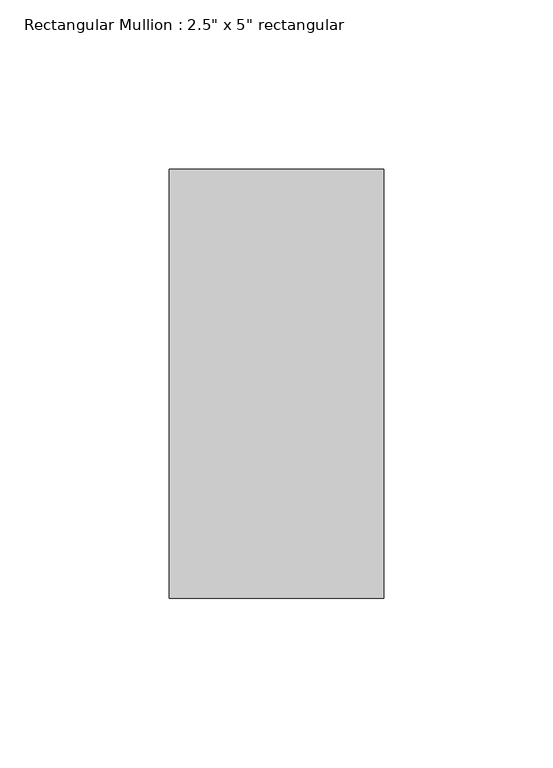
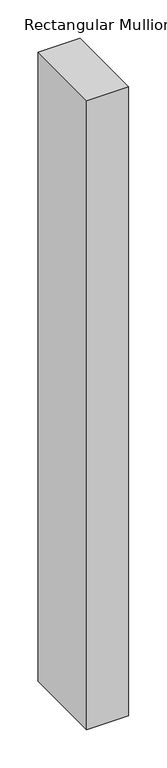
"""IFC4 building model written with IfcOpenShell, lengths in millimetres: member geometry."""

from ifc_helpers import new_model, si_unit, frame, origin, place, context, project, spatial, polyline, outline, extrude, source, transform, mapped, element, save


def member_cfcad22e(model_context):
    return source(origin(), model_context, "Body", "SweptSolid", [
        extrude(outline(polyline([(0.0, 63.5), (0.0, -63.5), (-63.5, -63.5), (-63.5, 63.5), (0.0, 63.5)])), frame((0.0, 0.0, -1003.3), z_axis=(0.0, 0.0, 1.0), x_axis=(1.0, 0.0, 0.0)), (0.0, 0.0, 1.0), 1003.3),
    ])


if __name__ == "__main__":
    model = new_model("IFC4")
    model_context = context("Model", 3, world=origin())
    ifc_project = project(units=[si_unit("LENGTHUNIT", "METRE", prefix="MILLI")], contexts=[model_context])
    site = spatial("IfcSite", under=ifc_project)
    building = spatial("IfcBuilding", under=site)
    placement = place(None, origin())
    member_shape = member_cfcad22e(model_context)
    element("IfcMember", 1, ObjectType="Rectangular Mullion : 2.5\" x 5\" rectangular", at=placement, inside=building, context=model_context, shape_type="MappedRepresentation", body=[
        mapped(member_shape, transform((0.0, 0.0, 0.0), x_axis=(1.0, 0.0, 0.0), y_axis=(0.0, 1.0, 0.0), z_axis=(0.0, 0.0, 1.0))),
    ])
    save(model, "model.ifc")

# Revit data of these elements
# Type "Rectangular Mullion : 2.5\" x 5\" rectangular"
#   built-in parameter 1007304 = 0.416667 (stored number, unit not read)
#   built-in parameter 1007301 = 0.104167 (stored number, unit not read)
#   built-in parameter 1007300 = 0.104167 (stored number, unit not read)
# Element 1 (IfcMember, "Rectangular Mullion : 2.5\" x 5\" rectangular")
#   Materials on its faces: "Aluminum"
# Materials
#   "Aluminum": class "Metal", colour RGB 247 247 247, transparency 0, Description = "Aluminum 6061", Cost = 0
